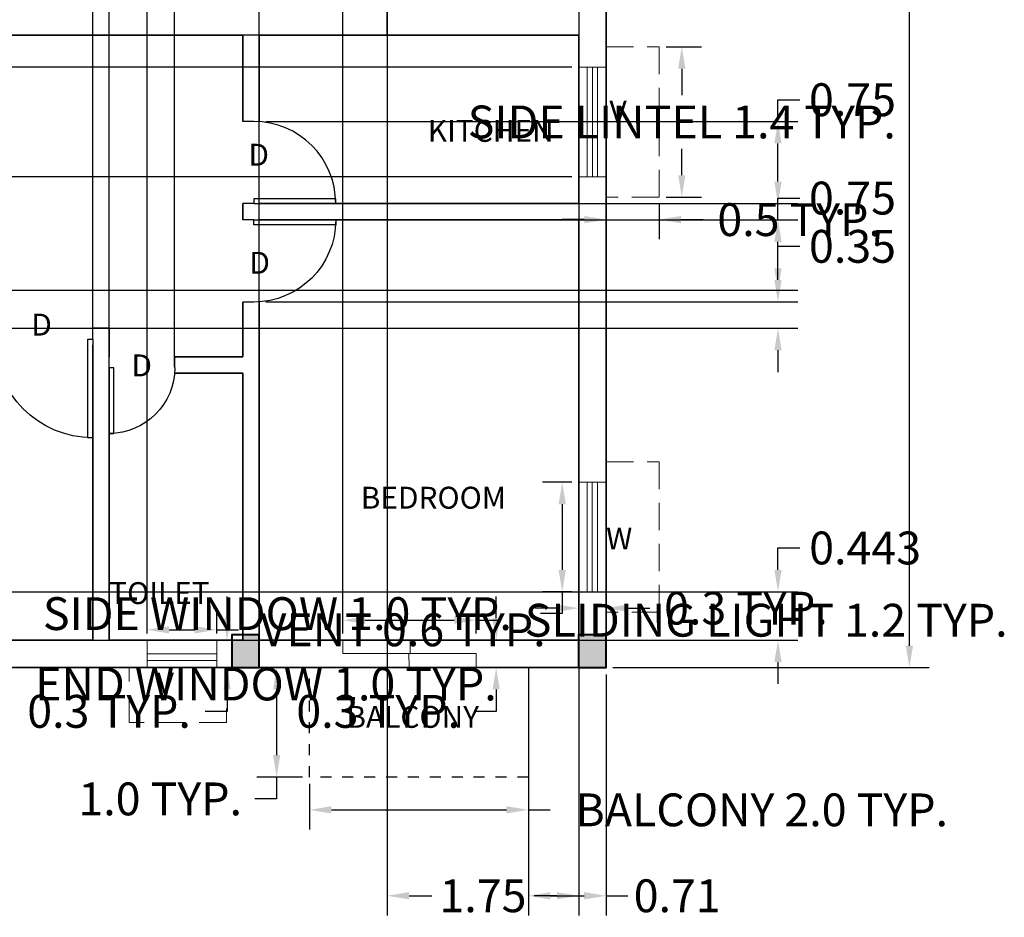
# Model space of a CAD drawing. Units: metres. Extents: x 106.5 to 121.4, y 89.1 to 111.8.
# Tile 2 of 5: x 112.4 to 121.4, y 89.1 to 97.3. Entities that reach past the tile are written whole.
import ezdxf

# ---------------------------------------------------------------- set-up
doc = ezdxf.new("R2010")
doc.units = ezdxf.units.M
doc.header["$MEASUREMENT"] = 0
doc.linetypes.add('ACAD_ISO07W100', pattern=[3, 0, -3])
doc.linetypes.add('HIDDEN', pattern=[0.375, 0.25, -0.125])
doc.layers.get('0').update_dxf_attribs({"color": 1})
for name, color, linetype, lineweight in [('A-ANNO-DIMS', 5, 'Continuous', 18), ('A-ANNO-TEXT', 4, 'Continuous', 18), ('A-AREA-IDEN', 4, 'Continuous', 18), ('A-COLS-PATT', 18, 'Continuous', 13), ('A-FLOR-BALC', 240, 'ACAD_ISO07W100', 25), ('A-WALL', 1, 'Continuous', 35), ('COLUMN', 244, 'Continuous', 40), ('DR', 2, 'Continuous', 25), ('LNTL', 240, 'HIDDEN', 18), ('VNTLTR', 8, 'Continuous', 18), ('WNDW', 3, 'Continuous', 18)]:
    doc.layers.add(name, color=color, linetype=linetype, lineweight=lineweight)
doc.styles.get("Standard").update_dxf_attribs({"font": 'arial.ttf'})
doc.dimstyles.get("Standard").update_dxf_attribs({"dimtxt": 0.3, "dimasz": 0.2, "dimexe": 0.18, "dimexo": 0.0625, "dimgap": 0.09, "dimtad": 0, "dimtih": 1, "dimtoh": 1, "dimdec": 1, "dimzin": 0, "dimdsep": 46, "dimtxsty": 'Standard', "dimcen": 0.09, "dimadec": 0, "dimazin": 0, "dimtfac": 1, "dimtdec": 1, "dimtofl": 0, "dimtmove": 0, "dimatfit": 3, "dimfxl": 1, "dimtolj": 1, "dimtzin": 0, "dimarcsym": 0})

# ---------------------------------------------------------------- blocks, each defined once
blk = doc.blocks.new('*U2')
for p, q in [((0, 0), (0, -100)), ((-900, 0), (-900, -100))]:
    blk.add_line(p, q)
blk.add_lwpolyline([(0, 0), (0, 900), (-43.75, 900), (-43.75, 0)], close=True)
blk.add_arc((0, 0), 900, 90, 180)
blk = doc.blocks.new('*U3')
for p, q in [((0, 0), (0, -100)), ((600, 0), (600, -100))]:
    blk.add_line(p, q)
blk.add_lwpolyline([(0, 0), (0, 600), (43.75, 600), (43.75, 0)], close=True)
blk.add_arc((0, 0), 600, 0, 90)
blk = doc.blocks.new('*U4')
for p, q in [((-750, 0), (-750, -100)), ((0, 0), (0, -100))]:
    blk.add_line(p, q)
blk.add_lwpolyline([(0, 0), (0, 750), (-43.75, 750), (-43.75, 0)], close=True)
blk.add_arc((0, 0), 750, 90, 180)
blk = doc.blocks.new('*D24')
at = {"layer": 'A-ANNO-DIMS', "color": 0, "lineweight": -2, "ltscale": 0.5, "transparency": 16777216}
for p, q in [((117.8454, 109.5038), (120.7343, 109.5038)), ((120.5543, 109.3038), (120.5543, 100.662)), ((120.5543, 91.5338), (120.5543, 100.1756)), ((117.8446, 91.3338), (120.7343, 91.3338))]:
    blk.add_line(p, q, dxfattribs=at)
at = {"layer": 'A-ANNO-DIMS', "color": 0, "lineweight": -3, "ltscale": 0.5, "transparency": 16777216}
for points in [[(120.521, 109.3038), (120.5876, 109.3038), (120.5543, 109.5038)], [(120.521, 91.5338), (120.5876, 91.5338), (120.5543, 91.3338)]]:
    blk.add_solid(points, dxfattribs=at)
at = {"layer": 'Defpoints', "color": 0, "lineweight": -3, "ltscale": 0.5, "transparency": 16777216}
for p in [(117.7829, 109.5038), (117.7821, 91.3338), (120.5543, 91.3338)]:
    blk.add_point(p, dxfattribs=at)
at = {"layer": 'A-ANNO-DIMS', "color": 0, "ltscale": 0.5, "transparency": 16777216, "insert": (120.5543, 100.4188), "char_height": 0.3, "attachment_point": 5}
blk.add_mtext('\\A1;18.2', dxfattribs=at)
blk = doc.blocks.new('WIN-1000-SIDE')
for p, q in [((0.0782, 0.9998), (0.0782, -0.0002)), ((0.1249, 0.9998), (0.1249, -0.0002)), ((0.1718, -0.0002), (0.1718, 0.9998))]:
    blk.add_line(p, q)
blk.add_lwpolyline([(-0.0001, 0.9998), (0.2499, 0.9998), (0.2499, -0.0002), (-0.0001, -0.0002)], close=True)
blk = doc.blocks.new('BALCONY-SLIDING-LIGHT')
for points in [[(0.6038, 0.2498), (1.217, 0.2498), (1.217, 0.1224), (0.6014, 0.1224)], [(-0.0001, -0.0002), (0.613, -0.0002), (0.613, 0.1224), (-0.0001, 0.1224)]]:
    blk.add_lwpolyline(points, close=True)
blk = doc.blocks.new('VENT-0634')
for p, q in [((-0.0005, 0.1839), (0.6339, 0.1839)), ((-0.0005, 0.1248), (0.6339, 0.1248))]:
    blk.add_line(p, q)
blk.add_lwpolyline([(-0.0005, 0.2498), (0.6339, 0.2498), (0.6339, -0.0002), (-0.0005, -0.0002)], close=True)
blk = doc.blocks.new('LINTEL-PROJ-1373')
for p, q in [((-0.0001, 1.3733), (0.4855, 1.3733)), ((0.4855, 1.3733), (0.4855, 0.0001)), ((0.4855, 0.0001), (-0.0001, 0.0001))]:
    blk.add_line(p, q)
blk = doc.blocks.new('LINTEL-PROJ-0890')
for p, q in [((0.0002, -0.0002), (0.0002, 0.5015)), ((0.0002, 0.5015), (0.8897, 0.5015)), ((0.8897, 0.5015), (0.8897, -0.0002))]:
    blk.add_line(p, q)
blk = doc.blocks.new('BALCONY-2000X1000')
at = {"ltscale": 0.02}
blk.add_lwpolyline([(-0.0001, -0.0002), (1.9999, -0.0002), (1.9999, 0.9998), (-0.0001, 0.9998)], close=True, dxfattribs=at)
blk = doc.blocks.new('COL-250X300')
at = {"ltscale": 0.5}
blk.add_lwpolyline([(-0.0001, 0.2999), (0.2499, 0.2999), (0.2499, -0.0001), (-0.0001, -0.0001)], close=True, dxfattribs=at)
blk = doc.blocks.new('*D38')
at = {"layer": 'A-ANNO-DIMS', "color": 0, "lineweight": -2, "ltscale": 0.5, "transparency": 16777216}
for p, q in [((117.4697, 93.0268), (117.2022, 93.0268)), ((117.3822, 92.8268), (117.3822, 92.2268)), ((117.4697, 92.0268), (117.2022, 92.0268)), ((117.3822, 92.0268), (117.3822, 91.8268)), ((117.3822, 91.8268), (117.1822, 91.8268))]:
    blk.add_line(p, q, dxfattribs=at)
at = {"layer": 'A-ANNO-DIMS', "color": 0, "lineweight": -3, "ltscale": 0.5, "transparency": 16777216}
for points in [[(117.3488, 92.8268), (117.4155, 92.8268), (117.3822, 93.0268)], [(117.3488, 92.2268), (117.4155, 92.2268), (117.3822, 92.0268)]]:
    blk.add_solid(points, dxfattribs=at)
at = {"layer": 'Defpoints', "color": 0, "lineweight": -3, "ltscale": 0.5, "transparency": 16777216}
for p in [(117.5322, 93.0268), (117.3822, 92.0268), (117.5322, 92.0268)]:
    blk.add_point(p, dxfattribs=at)
at = {"layer": 'A-ANNO-DIMS', "color": 0, "ltscale": 0.5, "transparency": 16777216, "insert": (114.7795, 91.8268), "char_height": 0.3, "attachment_point": 5}
blk.add_mtext('\\A1;SIDE WINDOW 1.0 TYP.', dxfattribs=at)
blk = doc.blocks.new('*D39')
at = {"layer": 'A-ANNO-DIMS', "color": 0, "lineweight": -2, "ltscale": 0.5, "transparency": 16777216}
for p, q in [((117.5322, 91.9643), (117.5322, 91.6968)), ((117.7822, 91.9643), (117.7822, 91.6968)), ((117.3322, 91.8768), (117.1322, 91.8768)), ((117.9822, 91.8768), (118.1822, 91.8768))]:
    blk.add_line(p, q, dxfattribs=at)
at = {"layer": 'A-ANNO-DIMS', "color": 0, "lineweight": -3, "ltscale": 0.5, "transparency": 16777216}
for points in [[(117.3322, 91.9101), (117.3322, 91.8434), (117.5322, 91.8768)], [(117.9822, 91.9101), (117.9822, 91.8434), (117.7822, 91.8768)]]:
    blk.add_solid(points, dxfattribs=at)
at = {"layer": 'Defpoints', "color": 0, "lineweight": -3, "ltscale": 0.5, "transparency": 16777216}
for p in [(117.5322, 92.0268), (117.7822, 92.0268), (117.7822, 91.8768)]:
    blk.add_point(p, dxfattribs=at)
at = {"layer": 'A-ANNO-DIMS', "color": 0, "ltscale": 0.5, "transparency": 16777216, "insert": (119.0605, 91.8768), "char_height": 0.3, "attachment_point": 5}
blk.add_mtext('\\A1;0.3 TYP.', dxfattribs=at)
blk = doc.blocks.new('*D40')
at = {"layer": 'A-ANNO-DIMS', "color": 0, "lineweight": -2, "ltscale": 0.5, "transparency": 16777216}
for p, q in [((111.1267, 91.2713), (111.1267, 91.0038)), ((112.1267, 91.2713), (112.1267, 91.0038)), ((111.3267, 91.1838), (111.9267, 91.1838)), ((112.1267, 91.1838), (112.3267, 91.1838))]:
    blk.add_line(p, q, dxfattribs=at)
at = {"layer": 'A-ANNO-DIMS', "color": 0, "lineweight": -3, "ltscale": 0.5, "transparency": 16777216}
for points in [[(111.3267, 91.2171), (111.3267, 91.1505), (111.1267, 91.1838)], [(111.9267, 91.2171), (111.9267, 91.1505), (112.1267, 91.1838)]]:
    blk.add_solid(points, dxfattribs=at)
at = {"layer": 'Defpoints', "color": 0, "lineweight": -3, "ltscale": 0.5, "transparency": 16777216}
for p in [(111.1267, 91.3338), (112.1267, 91.3338), (112.1267, 91.1838)]:
    blk.add_point(p, dxfattribs=at)
at = {"layer": 'A-ANNO-DIMS', "color": 0, "ltscale": 0.5, "transparency": 16777216, "insert": (114.6755, 91.1838), "char_height": 0.3, "attachment_point": 5}
blk.add_mtext('\\A1;END WINDOW 1.0 TYP.', dxfattribs=at)
blk = doc.blocks.new('*D44')
at = {"layer": 'A-ANNO-DIMS', "color": 0, "lineweight": -2, "ltscale": 0.5, "transparency": 16777216}
for p, q in [((115.3789, 91.6463), (115.3789, 91.9464)), ((116.596, 91.6463), (116.596, 91.9464)), ((115.5789, 91.7664), (116.396, 91.7664)), ((116.596, 91.7664), (116.796, 91.7664))]:
    blk.add_line(p, q, dxfattribs=at)
at = {"layer": 'A-ANNO-DIMS', "color": 0, "lineweight": -3, "ltscale": 0.5, "transparency": 16777216}
for points in [[(115.5789, 91.7997), (115.5789, 91.733), (115.3789, 91.7664)], [(116.396, 91.7997), (116.396, 91.733), (116.596, 91.7664)]]:
    blk.add_solid(points, dxfattribs=at)
at = {"layer": 'Defpoints', "color": 0, "lineweight": -3, "ltscale": 0.5, "transparency": 16777216}
for p in [(116.596, 91.7664), (115.3789, 91.5838), (116.596, 91.5838)]:
    blk.add_point(p, dxfattribs=at)
at = {"layer": 'A-ANNO-DIMS', "color": 0, "ltscale": 0.5, "transparency": 16777216, "insert": (119.2456, 91.7664), "char_height": 0.3, "attachment_point": 5}
blk.add_mtext('\\A1;SLIDING LIGHT 1.2 TYP.', dxfattribs=at)
blk = doc.blocks.new('*D45')
at = {"layer": 'A-ANNO-DIMS', "color": 0, "lineweight": -2, "ltscale": 0.5, "transparency": 16777216}
for p, q in [((116.7785, 91.7838), (116.7785, 91.9838)), ((116.6585, 91.5838), (116.9585, 91.5838)), ((116.6585, 91.3338), (116.9585, 91.3338)), ((116.7785, 91.1338), (116.7785, 90.9338)), ((116.7785, 90.9338), (116.5785, 90.9338))]:
    blk.add_line(p, q, dxfattribs=at)
at = {"layer": 'A-ANNO-DIMS', "color": 0, "lineweight": -3, "ltscale": 0.5, "transparency": 16777216}
for points in [[(116.7452, 91.7838), (116.8119, 91.7838), (116.7785, 91.5838)], [(116.7452, 91.1338), (116.8119, 91.1338), (116.7785, 91.3338)]]:
    blk.add_solid(points, dxfattribs=at)
at = {"layer": 'Defpoints', "color": 0, "lineweight": -3, "ltscale": 0.5, "transparency": 16777216}
for p in [(116.596, 91.5838), (116.596, 91.3338), (116.7785, 91.3338)]:
    blk.add_point(p, dxfattribs=at)
at = {"layer": 'A-ANNO-DIMS', "color": 0, "ltscale": 0.5, "transparency": 16777216, "insert": (115.7002, 90.9338), "char_height": 0.3, "attachment_point": 5}
blk.add_mtext('\\A1;0.3 TYP.', dxfattribs=at)
blk = doc.blocks.new('*D46')
at = {"layer": 'A-ANNO-DIMS', "color": 0, "lineweight": -2, "ltscale": 0.5, "transparency": 16777216}
for p, q in [((113.5905, 91.6463), (113.5905, 91.859)), ((114.2249, 91.6463), (114.2249, 91.859)), ((113.7905, 91.679), (114.0249, 91.679)), ((114.2249, 91.679), (114.4249, 91.679))]:
    blk.add_line(p, q, dxfattribs=at)
at = {"layer": 'A-ANNO-DIMS', "color": 0, "lineweight": -3, "ltscale": 0.5, "transparency": 16777216}
for points in [[(113.7905, 91.7123), (113.7905, 91.6456), (113.5905, 91.679)], [(114.0249, 91.7123), (114.0249, 91.6456), (114.2249, 91.679)]]:
    blk.add_solid(points, dxfattribs=at)
at = {"layer": 'Defpoints', "color": 0, "lineweight": -3, "ltscale": 0.5, "transparency": 16777216}
for p in [(114.2249, 91.679), (113.5905, 91.5838), (114.2249, 91.5838)]:
    blk.add_point(p, dxfattribs=at)
at = {"layer": 'A-ANNO-DIMS', "color": 0, "ltscale": 0.5, "transparency": 16777216, "insert": (115.9281, 91.679), "char_height": 0.3, "attachment_point": 5}
blk.add_mtext('\\A1;VENT 0.6 TYP.', dxfattribs=at)
blk = doc.blocks.new('*D47')
at = {"layer": 'A-ANNO-DIMS', "color": 0, "lineweight": -2, "ltscale": 0.5, "transparency": 16777216}
for p, q in [((114.32, 91.7838), (114.32, 91.9838)), ((114.2874, 91.5838), (114.5, 91.5838)), ((114.2874, 91.3338), (114.5, 91.3338)), ((114.32, 91.1338), (114.32, 90.9338)), ((114.32, 90.9338), (114.12, 90.9338))]:
    blk.add_line(p, q, dxfattribs=at)
at = {"layer": 'A-ANNO-DIMS', "color": 0, "lineweight": -3, "ltscale": 0.5, "transparency": 16777216}
for points in [[(114.2867, 91.7838), (114.3534, 91.7838), (114.32, 91.5838)], [(114.2867, 91.1338), (114.3534, 91.1338), (114.32, 91.3338)]]:
    blk.add_solid(points, dxfattribs=at)
at = {"layer": 'Defpoints', "color": 0, "lineweight": -3, "ltscale": 0.5, "transparency": 16777216}
for p in [(114.2249, 91.5838), (114.2249, 91.3338), (114.32, 91.3338)]:
    blk.add_point(p, dxfattribs=at)
at = {"layer": 'A-ANNO-DIMS', "color": 0, "ltscale": 0.5, "transparency": 16777216, "insert": (113.2417, 90.9338), "char_height": 0.3, "attachment_point": 5}
blk.add_mtext('\\A1;0.3 TYP.', dxfattribs=at)
blk = doc.blocks.new('*D50')
at = {"layer": 'A-ANNO-DIMS', "color": 0, "lineweight": -2, "ltscale": 0.5, "transparency": 16777216}
for p, q in [((118.331, 97.0058), (118.6544, 97.0058)), ((118.4744, 96.8058), (118.4744, 96.5644)), ((118.4744, 95.8327), (118.4744, 96.0742)), ((118.331, 95.6327), (118.6544, 95.6327))]:
    blk.add_line(p, q, dxfattribs=at)
at = {"layer": 'A-ANNO-DIMS', "color": 0, "lineweight": -3, "ltscale": 0.5, "transparency": 16777216}
for points in [[(118.4411, 96.8058), (118.5078, 96.8058), (118.4744, 97.0058)], [(118.4411, 95.8327), (118.5078, 95.8327), (118.4744, 95.6327)]]:
    blk.add_solid(points, dxfattribs=at)
at = {"layer": 'Defpoints', "color": 0, "lineweight": -3, "ltscale": 0.5, "transparency": 16777216}
for p in [(118.2685, 97.0058), (118.4744, 97.0058), (118.2685, 95.6327)]:
    blk.add_point(p, dxfattribs=at)
at = {"layer": 'A-ANNO-DIMS', "color": 0, "ltscale": 0.5, "transparency": 16777216, "insert": (118.4744, 96.3193), "char_height": 0.3, "attachment_point": 5}
blk.add_mtext('\\A1;SIDE LINTEL 1.4 TYP.', dxfattribs=at)
blk = doc.blocks.new('*D51')
at = {"layer": 'A-ANNO-DIMS', "color": 0, "lineweight": -2, "ltscale": 0.5, "transparency": 16777216}
for p, q in [((117.7829, 95.5702), (117.7829, 95.2468)), ((118.2685, 95.5702), (118.2685, 95.2468)), ((117.5829, 95.4268), (117.3829, 95.4268)), ((118.4685, 95.4268), (118.6685, 95.4268))]:
    blk.add_line(p, q, dxfattribs=at)
at = {"layer": 'A-ANNO-DIMS', "color": 0, "lineweight": -3, "ltscale": 0.5, "transparency": 16777216}
for points in [[(117.5829, 95.4601), (117.5829, 95.3934), (117.7829, 95.4268)], [(118.4685, 95.4601), (118.4685, 95.3934), (118.2685, 95.4268)]]:
    blk.add_solid(points, dxfattribs=at)
at = {"layer": 'Defpoints', "color": 0, "lineweight": -3, "ltscale": 0.5, "transparency": 16777216}
for p in [(117.7829, 95.6327), (118.2685, 95.6327), (118.2685, 95.4268)]:
    blk.add_point(p, dxfattribs=at)
at = {"layer": 'A-ANNO-DIMS', "color": 0, "ltscale": 0.5, "transparency": 16777216, "insert": (119.5468, 95.4268), "char_height": 0.3, "attachment_point": 5}
blk.add_mtext('\\A1;0.5 TYP.', dxfattribs=at)
blk = doc.blocks.new('*D56')
at = {"layer": 'A-ANNO-DIMS', "color": 0, "lineweight": -2, "ltscale": 0.5, "transparency": 16777216}
for p, q in [((115.0729, 90.2713), (115.0729, 89.8538)), ((117.0729, 90.2713), (117.0729, 89.8538)), ((115.2729, 90.0338), (116.8729, 90.0338)), ((117.0729, 90.0338), (117.2729, 90.0338))]:
    blk.add_line(p, q, dxfattribs=at)
at = {"layer": 'A-ANNO-DIMS', "color": 0, "lineweight": -3, "ltscale": 0.5, "transparency": 16777216}
for points in [[(115.2729, 90.0671), (115.2729, 90.0005), (115.0729, 90.0338)], [(116.8729, 90.0671), (116.8729, 90.0005), (117.0729, 90.0338)]]:
    blk.add_solid(points, dxfattribs=at)
at = {"layer": 'Defpoints', "color": 0, "lineweight": -3, "ltscale": 0.5, "transparency": 16777216}
for p in [(115.0729, 90.3338), (117.0729, 90.3338), (117.0729, 90.0338)]:
    blk.add_point(p, dxfattribs=at)
at = {"layer": 'A-ANNO-DIMS', "color": 0, "ltscale": 0.5, "transparency": 16777216, "insert": (119.2044, 90.0338), "char_height": 0.3, "attachment_point": 5}
blk.add_mtext('\\A1;BALCONY 2.0 TYP.', dxfattribs=at)
blk = doc.blocks.new('*D57')
at = {"layer": 'A-ANNO-DIMS', "color": 0, "lineweight": -2, "ltscale": 0.5, "transparency": 16777216}
for p, q in [((115.0104, 91.3338), (114.5929, 91.3338)), ((114.7729, 91.1338), (114.7729, 90.5338)), ((115.0104, 90.3338), (114.5929, 90.3338)), ((114.7729, 90.3338), (114.7729, 90.1338)), ((114.7729, 90.1338), (114.5729, 90.1338))]:
    blk.add_line(p, q, dxfattribs=at)
at = {"layer": 'A-ANNO-DIMS', "color": 0, "lineweight": -3, "ltscale": 0.5, "transparency": 16777216}
for points in [[(114.7396, 91.1338), (114.8063, 91.1338), (114.7729, 91.3338)], [(114.7396, 90.5338), (114.8063, 90.5338), (114.7729, 90.3338)]]:
    blk.add_solid(points, dxfattribs=at)
at = {"layer": 'Defpoints', "color": 0, "lineweight": -3, "ltscale": 0.5, "transparency": 16777216}
for p in [(115.0729, 91.3338), (114.7729, 90.3338), (115.0729, 90.3338)]:
    blk.add_point(p, dxfattribs=at)
at = {"layer": 'A-ANNO-DIMS', "color": 0, "ltscale": 0.5, "transparency": 16777216, "insert": (113.7087, 90.1338), "char_height": 0.3, "attachment_point": 5}
blk.add_mtext('\\A1;1.0 TYP.', dxfattribs=at)
blk = doc.blocks.new('*D59')
at = {"layer": 'A-ANNO-DIMS', "color": 0, "lineweight": -2, "ltscale": 0.5, "transparency": 16777216}
for p, q in [((112.1943, 94.3463), (112.1943, 111.7688)), ((113.0929, 94.3463), (113.0929, 111.7688)), ((112.3943, 111.5888), (112.8929, 111.5888)), ((113.0929, 111.5888), (113.2929, 111.5888))]:
    blk.add_line(p, q, dxfattribs=at)
at = {"layer": 'A-ANNO-DIMS', "color": 0, "lineweight": -3, "ltscale": 0.5, "transparency": 16777216}
for points in [[(112.3943, 111.6221), (112.3943, 111.5555), (112.1943, 111.5888)], [(112.8929, 111.6221), (112.8929, 111.5555), (113.0929, 111.5888)]]:
    blk.add_solid(points, dxfattribs=at)
at = {"layer": 'Defpoints', "color": 0, "lineweight": -3, "ltscale": 0.5, "transparency": 16777216}
for p in [(113.0929, 111.5888), (112.1943, 94.2838), (113.0929, 94.2838)]:
    blk.add_point(p, dxfattribs=at)
at = {"layer": 'A-ANNO-DIMS', "color": 0, "ltscale": 0.5, "transparency": 16777216, "insert": (113.772, 111.5888), "char_height": 0.3, "attachment_point": 5}
blk.add_mtext('\\A1;0.90', dxfattribs=at)
blk = doc.blocks.new('*D60')
at = {"layer": 'A-ANNO-DIMS', "color": 0, "lineweight": -2, "ltscale": 0.5, "transparency": 16777216}
for p, q in [((113.2429, 94.0863), (113.2429, 111.7688)), ((113.8408, 94.0863), (113.8408, 111.7688)), ((113.4429, 111.5888), (113.6408, 111.5888)), ((113.8408, 111.5888), (114.0408, 111.5888))]:
    blk.add_line(p, q, dxfattribs=at)
at = {"layer": 'A-ANNO-DIMS', "color": 0, "lineweight": -3, "ltscale": 0.5, "transparency": 16777216}
for points in [[(113.4429, 111.6221), (113.4429, 111.5555), (113.2429, 111.5888)], [(113.6408, 111.6221), (113.6408, 111.5555), (113.8408, 111.5888)]]:
    blk.add_solid(points, dxfattribs=at)
at = {"layer": 'Defpoints', "color": 0, "lineweight": -3, "ltscale": 0.5, "transparency": 16777216}
for p in [(113.8408, 111.5888), (113.2429, 94.0238), (113.8408, 94.0238)]:
    blk.add_point(p, dxfattribs=at)
at = {"layer": 'A-ANNO-DIMS', "color": 0, "ltscale": 0.5, "transparency": 16777216, "insert": (114.6373, 111.5888), "char_height": 0.3, "attachment_point": 5}
blk.add_mtext('\\A1;0.598', dxfattribs=at)
blk = doc.blocks.new('*D61')
at = {"layer": 'A-ANNO-DIMS', "color": 0, "lineweight": -2, "ltscale": 0.5, "transparency": 16777216}
for p, q in [((119.3535, 95.4238), (119.3535, 95.6238)), ((119.3535, 95.6238), (119.5535, 95.6238)), ((114.6754, 95.4238), (119.5335, 95.4238)), ((119.3535, 94.8755), (119.3535, 95.2238)), ((114.6754, 94.6755), (119.5335, 94.6755))]:
    blk.add_line(p, q, dxfattribs=at)
at = {"layer": 'A-ANNO-DIMS', "color": 0, "lineweight": -3, "ltscale": 0.5, "transparency": 16777216}
for points in [[(119.3201, 95.2238), (119.3868, 95.2238), (119.3535, 95.4238)], [(119.3201, 94.8755), (119.3868, 94.8755), (119.3535, 94.6755)]]:
    blk.add_solid(points, dxfattribs=at)
at = {"layer": 'Defpoints', "color": 0, "lineweight": -3, "ltscale": 0.5, "transparency": 16777216}
for p in [(114.6129, 95.4238), (119.3535, 95.4238), (114.6129, 94.6755)]:
    blk.add_point(p, dxfattribs=at)
at = {"layer": 'A-ANNO-DIMS', "color": 0, "ltscale": 0.5, "transparency": 16777216, "insert": (120.0342, 95.6238), "char_height": 0.3, "attachment_point": 5}
blk.add_mtext('\\A1;0.75', dxfattribs=at)
blk = doc.blocks.new('*D62')
at = {"layer": 'A-ANNO-DIMS', "color": 0, "lineweight": -2, "ltscale": 0.5, "transparency": 16777216}
for p, q in [((119.3535, 96.3225), (119.3535, 96.5225)), ((119.3535, 96.5225), (119.5535, 96.5225)), ((114.6754, 96.3225), (119.5335, 96.3225)), ((119.3535, 95.7738), (119.3535, 96.1225)), ((114.6754, 95.5738), (119.5335, 95.5738))]:
    blk.add_line(p, q, dxfattribs=at)
at = {"layer": 'A-ANNO-DIMS', "color": 0, "lineweight": -3, "ltscale": 0.5, "transparency": 16777216}
for points in [[(119.3201, 96.1225), (119.3868, 96.1225), (119.3535, 96.3225)], [(119.3201, 95.7738), (119.3868, 95.7738), (119.3535, 95.5738)]]:
    blk.add_solid(points, dxfattribs=at)
at = {"layer": 'Defpoints', "color": 0, "lineweight": -3, "ltscale": 0.5, "transparency": 16777216}
for p in [(114.6129, 96.3225), (119.3535, 96.3225), (114.6129, 95.5738)]:
    blk.add_point(p, dxfattribs=at)
at = {"layer": 'A-ANNO-DIMS', "color": 0, "ltscale": 0.5, "transparency": 16777216, "insert": (120.0342, 96.5225), "char_height": 0.3, "attachment_point": 5}
blk.add_mtext('\\A1;0.75', dxfattribs=at)
blk = doc.blocks.new('*D64')
at = {"layer": 'A-ANNO-DIMS', "color": 0, "lineweight": -2, "ltscale": 0.5, "transparency": 16777216}
for p, q in [((113.2429, 91.6463), (113.2429, 111.7688)), ((113.5905, 91.6463), (113.5905, 111.7688)), ((113.0429, 111.5888), (112.8429, 111.5888)), ((113.7905, 111.5888), (113.9905, 111.5888))]:
    blk.add_line(p, q, dxfattribs=at)
at = {"layer": 'A-ANNO-DIMS', "color": 0, "lineweight": -3, "ltscale": 0.5, "transparency": 16777216}
for points in [[(113.0429, 111.6221), (113.0429, 111.5555), (113.2429, 111.5888)], [(113.7905, 111.6221), (113.7905, 111.5555), (113.5905, 111.5888)]]:
    blk.add_solid(points, dxfattribs=at)
at = {"layer": 'Defpoints', "color": 0, "lineweight": -3, "ltscale": 0.5, "transparency": 16777216}
for p in [(113.5905, 111.5888), (113.2429, 91.5838), (113.5905, 91.5838)]:
    blk.add_point(p, dxfattribs=at)
at = {"layer": 'A-ANNO-DIMS', "color": 0, "ltscale": 0.5, "transparency": 16777216, "insert": (114.4713, 111.5888), "char_height": 0.3, "attachment_point": 5}
blk.add_mtext('\\A1;0.35', dxfattribs=at)
blk = doc.blocks.new('*D65')
at = {"layer": 'A-ANNO-DIMS', "color": 0, "lineweight": -2, "ltscale": 0.5, "transparency": 16777216}
for p, q in [((114.6129, 91.6463), (114.6129, 111.7688)), ((115.3789, 91.6463), (115.3789, 111.7688)), ((114.8129, 111.5888), (115.1789, 111.5888)), ((115.3789, 111.5888), (115.5789, 111.5888))]:
    blk.add_line(p, q, dxfattribs=at)
at = {"layer": 'A-ANNO-DIMS', "color": 0, "lineweight": -3, "ltscale": 0.5, "transparency": 16777216}
for points in [[(114.8129, 111.6221), (114.8129, 111.5555), (114.6129, 111.5888)], [(115.1789, 111.6221), (115.1789, 111.5555), (115.3789, 111.5888)]]:
    blk.add_solid(points, dxfattribs=at)
at = {"layer": 'Defpoints', "color": 0, "lineweight": -3, "ltscale": 0.5, "transparency": 16777216}
for p in [(115.3789, 111.5888), (114.6129, 91.5838), (115.3789, 91.5838)]:
    blk.add_point(p, dxfattribs=at)
at = {"layer": 'A-ANNO-DIMS', "color": 0, "ltscale": 0.5, "transparency": 16777216, "insert": (116.1749, 111.5888), "char_height": 0.3, "attachment_point": 5}
blk.add_mtext('\\A1;0.766', dxfattribs=at)
blk = doc.blocks.new('*D66')
at = {"layer": 'A-ANNO-DIMS', "color": 0, "lineweight": -2, "ltscale": 0.5, "transparency": 16777216}
for p, q in [((117.0729, 91.2713), (117.0729, 89.0688)), ((117.7821, 91.2713), (117.7821, 89.0688)), ((117.2729, 89.2488), (117.5821, 89.2488)), ((117.7821, 89.2488), (117.9821, 89.2488))]:
    blk.add_line(p, q, dxfattribs=at)
at = {"layer": 'A-ANNO-DIMS', "color": 0, "lineweight": -3, "ltscale": 0.5, "transparency": 16777216}
for points in [[(117.2729, 89.2821), (117.2729, 89.2155), (117.0729, 89.2488)], [(117.5821, 89.2821), (117.5821, 89.2155), (117.7821, 89.2488)]]:
    blk.add_solid(points, dxfattribs=at)
at = {"layer": 'Defpoints', "color": 0, "lineweight": -3, "ltscale": 0.5, "transparency": 16777216}
for p in [(117.0729, 91.3338), (117.7821, 91.3338), (117.7821, 89.2488)]:
    blk.add_point(p, dxfattribs=at)
at = {"layer": 'A-ANNO-DIMS', "color": 0, "ltscale": 0.5, "transparency": 16777216, "insert": (118.4328, 89.2488), "char_height": 0.3, "attachment_point": 5}
blk.add_mtext('\\A1;0.71', dxfattribs=at)
blk = doc.blocks.new('*D67')
at = {"layer": 'A-ANNO-DIMS', "color": 0, "lineweight": -2, "ltscale": 0.5, "transparency": 16777216}
for p, q in [((119.3535, 92.2268), (119.3535, 92.4268)), ((119.3535, 92.4268), (119.5535, 92.4268)), ((110.5154, 92.0268), (119.5335, 92.0268)), ((110.5154, 91.5838), (119.5335, 91.5838)), ((119.3535, 91.3838), (119.3535, 91.1838))]:
    blk.add_line(p, q, dxfattribs=at)
at = {"layer": 'A-ANNO-DIMS', "color": 0, "lineweight": -3, "ltscale": 0.5, "transparency": 16777216}
for points in [[(119.3201, 92.2268), (119.3868, 92.2268), (119.3535, 92.0268)], [(119.3201, 91.3838), (119.3868, 91.3838), (119.3535, 91.5838)]]:
    blk.add_solid(points, dxfattribs=at)
at = {"layer": 'Defpoints', "color": 0, "lineweight": -3, "ltscale": 0.5, "transparency": 16777216}
for p in [(110.4529, 92.0268), (119.3535, 92.0268), (110.4529, 91.5838)]:
    blk.add_point(p, dxfattribs=at)
at = {"layer": 'A-ANNO-DIMS', "color": 0, "ltscale": 0.5, "transparency": 16777216, "insert": (120.1496, 92.4268), "char_height": 0.3, "attachment_point": 5}
blk.add_mtext('\\A1;0.443', dxfattribs=at)
blk = doc.blocks.new('*D68')
at = {"layer": 'A-ANNO-DIMS', "color": 0, "lineweight": -2, "ltscale": 0.5, "transparency": 16777216}
for p, q in [((119.3535, 94.9829), (119.3535, 95.1829)), ((119.3535, 95.1829), (119.5535, 95.1829)), ((110.5154, 94.7829), (119.5335, 94.7829)), ((110.5154, 94.4338), (119.5335, 94.4338)), ((119.3535, 94.2338), (119.3535, 94.0338))]:
    blk.add_line(p, q, dxfattribs=at)
at = {"layer": 'A-ANNO-DIMS', "color": 0, "lineweight": -3, "ltscale": 0.5, "transparency": 16777216}
for points in [[(119.3201, 94.9829), (119.3868, 94.9829), (119.3535, 94.7829)], [(119.3201, 94.2338), (119.3868, 94.2338), (119.3535, 94.4338)]]:
    blk.add_solid(points, dxfattribs=at)
at = {"layer": 'Defpoints', "color": 0, "lineweight": -3, "ltscale": 0.5, "transparency": 16777216}
for p in [(110.4529, 94.7829), (119.3535, 94.7829), (110.4529, 94.4338)]:
    blk.add_point(p, dxfattribs=at)
at = {"layer": 'A-ANNO-DIMS', "color": 0, "ltscale": 0.5, "transparency": 16777216, "insert": (120.0342, 95.1829), "char_height": 0.3, "attachment_point": 5}
blk.add_mtext('\\A1;0.35', dxfattribs=at)
blk = doc.blocks.new('*D69')
at = {"layer": 'A-ANNO-DIMS', "color": 0, "lineweight": -2, "ltscale": 0.5, "transparency": 16777216}
for p, q in [((108.4073, 97.3137), (108.4073, 97.5137)), ((108.4073, 97.5137), (108.6073, 97.5137)), ((117.4704, 97.1137), (108.2273, 97.1137)), ((117.4697, 96.8192), (108.2273, 96.8192)), ((108.4073, 96.6192), (108.4073, 96.4192))]:
    blk.add_line(p, q, dxfattribs=at)
at = {"layer": 'A-ANNO-DIMS', "color": 0, "lineweight": -3, "ltscale": 0.5, "transparency": 16777216}
for points in [[(108.3739, 97.3137), (108.4406, 97.3137), (108.4073, 97.1137)], [(108.3739, 96.6192), (108.4406, 96.6192), (108.4073, 96.8192)]]:
    blk.add_solid(points, dxfattribs=at)
at = {"layer": 'Defpoints', "color": 0, "lineweight": -3, "ltscale": 0.5, "transparency": 16777216}
for p in [(108.4073, 97.1137), (117.5329, 97.1137), (117.5322, 96.8192)]:
    blk.add_point(p, dxfattribs=at)
at = {"layer": 'A-ANNO-DIMS', "color": 0, "ltscale": 0.5, "transparency": 16777216, "insert": (109.0872, 97.5137), "char_height": 0.3, "attachment_point": 5}
blk.add_mtext('\\A1;0.29', dxfattribs=at)
blk = doc.blocks.new('*D70')
at = {"layer": 'A-ANNO-DIMS', "color": 0, "lineweight": -2, "ltscale": 0.5, "transparency": 16777216}
for p, q in [((108.4073, 96.8192), (108.4073, 97.0191)), ((108.4073, 97.0191), (108.6073, 97.0191)), ((117.4697, 96.8192), (108.2273, 96.8192)), ((108.4073, 96.0192), (108.4073, 96.6192)), ((117.4697, 95.8192), (108.2273, 95.8192))]:
    blk.add_line(p, q, dxfattribs=at)
at = {"layer": 'A-ANNO-DIMS', "color": 0, "lineweight": -3, "ltscale": 0.5, "transparency": 16777216}
for points in [[(108.3739, 96.6192), (108.4406, 96.6192), (108.4073, 96.8192)], [(108.3739, 96.0192), (108.4406, 96.0192), (108.4073, 95.8192)]]:
    blk.add_solid(points, dxfattribs=at)
at = {"layer": 'Defpoints', "color": 0, "lineweight": -3, "ltscale": 0.5, "transparency": 16777216}
for p in [(108.4073, 96.8192), (117.5322, 96.8192), (117.5322, 95.8192)]:
    blk.add_point(p, dxfattribs=at)
at = {"layer": 'A-ANNO-DIMS', "color": 0, "ltscale": 0.5, "transparency": 16777216, "insert": (108.9557, 97.0191), "char_height": 0.3, "attachment_point": 5}
blk.add_mtext('\\A1;1.0', dxfattribs=at)
blk = doc.blocks.new('*D74')
at = {"layer": 'A-ANNO-DIMS', "color": 0, "lineweight": -2, "ltscale": 0.5, "transparency": 16777216}
for p, q in [((115.7829, 98.6813), (115.7829, 89.0688)), ((117.5329, 98.6813), (117.5329, 89.0688)), ((115.9829, 89.2488), (116.1913, 89.2488)), ((117.3329, 89.2488), (117.1246, 89.2488))]:
    blk.add_line(p, q, dxfattribs=at)
at = {"layer": 'A-ANNO-DIMS', "color": 0, "lineweight": -3, "ltscale": 0.5, "transparency": 16777216}
for points in [[(115.9829, 89.2821), (115.9829, 89.2155), (115.7829, 89.2488)], [(117.3329, 89.2821), (117.3329, 89.2155), (117.5329, 89.2488)]]:
    blk.add_solid(points, dxfattribs=at)
at = {"layer": 'Defpoints', "color": 0, "lineweight": -3, "ltscale": 0.5, "transparency": 16777216}
for p in [(115.7829, 98.7438), (117.5329, 98.7438), (117.5329, 89.2488)]:
    blk.add_point(p, dxfattribs=at)
at = {"layer": 'A-ANNO-DIMS', "color": 0, "ltscale": 0.5, "transparency": 16777216, "insert": (116.6579, 89.2488), "char_height": 0.3, "attachment_point": 5}
blk.add_mtext('\\A1;1.75', dxfattribs=at)

msp = doc.modelspace()

# ---------------------------------------------------------------- hatches: boundary and pattern name
at = {"layer": 'A-COLS-PATT', "ltscale": 0.5}
h = msp.add_hatch(color=256, dxfattribs=at)
h.dxf.hatch_style = 1
h.paths.add_polyline_path([(110.4529, 103.8929), (110.2029, 103.8929), (110.2029, 103.5938), (110.4529, 103.5938)])
h.paths.add_polyline_path([(114.4629, 103.8938), (114.3632, 103.8938), (114.3632, 103.7438), (114.4629, 103.7438)])
h.paths.add_polyline_path([(114.6129, 103.8938), (114.4629, 103.8938), (114.4629, 103.7438), (114.6129, 103.7438)])
h.paths.add_polyline_path([(114.6132, 103.7438), (114.4629, 103.7438), (114.3632, 103.7438), (114.3632, 103.5938), (114.6132, 103.5938)])
h.paths.add_polyline_path([(117.7829, 103.8996), (117.5329, 103.8996), (117.5329, 103.5996), (117.7829, 103.5996)])
h.paths.add_polyline_path([(117.7829, 98.888), (117.5329, 98.888), (117.5329, 98.588), (117.7829, 98.588)])
h.paths.add_polyline_path([(110.4529, 98.8938), (110.2029, 98.8938), (110.2029, 98.5947), (110.4529, 98.5947)])
h.paths.add_polyline_path([(114.6132, 98.8938), (114.3132, 98.8938), (114.3132, 98.7438), (114.4632, 98.7438), (114.6132, 98.7438)])
h.paths.add_polyline_path([(110.4529, 91.6338), (110.2029, 91.6338), (110.2029, 91.3338), (110.4529, 91.3338)])
h.paths.add_polyline_path([(114.6132, 91.5838), (114.6129, 91.5838), (114.6129, 91.6338), (114.4629, 91.6338), (114.4629, 91.5838), (114.3632, 91.5838), (114.3632, 91.3338), (114.6132, 91.3338)])
h.paths.add_polyline_path([(117.7821, 91.6338), (117.5329, 91.6338), (117.5329, 91.5838), (117.5321, 91.3338), (117.7821, 91.3338)])
h = msp.add_hatch(dxfattribs=at)
h.set_pattern_fill('CORK', color=256, scale=10)
h.set_pattern_definition([(0, (0, 0), (0, 1.25), []), (135, (0.625, -0.625), (-2.5, -2.5), [1.76777, -1.76777]), (135, (0.9375, -0.625), (-2.5, -2.5), [1.76777, -1.76777]), (135, (1.25, -0.625), (-2.5, -2.5), [1.76777, -1.76777])])
h.paths.add_polyline_path([(110.2029, 93.2238), (110.2029, 93.5238), (110.4529, 93.5238), (110.4529, 93.2238)])
h.paths.add_polyline_path([(114.6132, 93.2238), (114.3632, 93.2238), (114.3632, 93.4738), (114.4629, 93.4738), (114.4629, 93.5238), (114.6129, 93.5238), (114.6129, 93.4738)])
h.paths.add_polyline_path([(117.5321, 93.4738), (117.5329, 93.4738), (117.5329, 93.5238), (117.7821, 93.5238), (117.7821, 93.2238), (117.5321, 93.2238)])

# ---------------------------------------------------------------- linework, layer by layer
at = {"layer": 'A-WALL'}
for p, q in [((117.7829, 101.9438), (117.7829, 91.3338)), ((115.7829, 98.8938), (115.7829, 97.1137)), ((114.4629, 97.1137), (111.4529, 97.1137)), ((114.4629, 96.3242), (114.4629, 97.1137)), ((114.6129, 96.3225), (114.6129, 97.1137)), ((117.5329, 97.1137), (114.6129, 97.1137)), ((117.5329, 97.1137), (117.5329, 95.5738)), ((114.4629, 95.4238), (114.4629, 95.5742)), ((114.6129, 95.5738), (114.6129, 95.5742)), ((117.5329, 95.5738), (114.6129, 95.5738)), ((117.5329, 95.4238), (114.6129, 95.4238)), ((117.5329, 95.4238), (117.5329, 91.5838)), ((114.4629, 94.1738), (114.4629, 94.6738)), ((114.6129, 91.5838), (114.6129, 94.6755)), ((113.2429, 94.1738), (113.2429, 94.4338)), ((113.0929, 91.5838), (113.0929, 94.2838)), ((114.4629, 94.1738), (113.8429, 94.1738)), ((113.2429, 91.5838), (113.2429, 94.0238)), ((114.4629, 94.0238), (113.8408, 94.0238)), ((114.4629, 91.5838), (114.4629, 94.0238)), ((117.5322, 92.7838), (117.5329, 92.7838)), ((117.5322, 92.5338), (117.5329, 92.5338)), ((117.7822, 92.5338), (117.7829, 92.5338)), ((113.0929, 91.5838), (110.4529, 91.5838)), ((114.4629, 91.5838), (113.2429, 91.5838)), ((117.5329, 91.5838), (114.6129, 91.5838)), ((117.7829, 91.3338), (110.2029, 91.3338))]:
    msp.add_line(p, q, dxfattribs=at)
at = {"layer": 'A-WALL', "ltscale": 0.5}
msp.add_line((113.0929, 94.4338), (113.2429, 94.4338), dxfattribs=at)
msp.add_line((113.0929, 94.4338), (113.2429, 94.4338), dxfattribs=at)
at = {"layer": 'COLUMN', "ltscale": 0.5}
msp.add_lwpolyline([(117.5321, 91.3338), (117.7821, 91.3338), (117.7821, 91.6338), (117.5321, 91.6338)], close=True, dxfattribs=at)
at = {"layer": 'VNTLTR'}
for p, q in [((117.6105, 95.8191), (117.6105, 96.8191)), ((117.6572, 95.8191), (117.6572, 96.8191)), ((117.704, 96.8191), (117.704, 95.8191))]:
    msp.add_line(p, q, dxfattribs=at)
msp.add_lwpolyline([(117.5322, 95.8191), (117.7822, 95.8191), (117.7822, 96.8191), (117.5322, 96.8191)], close=True, dxfattribs=at)

# ---------------------------------------------------------------- block references
at = {"layer": 'A-FLOR-BALC', "extrusion": (0, 0, -1), "zscale": -1, "rotation": 180}
msp.add_blockref('BALCONY-2000X1000', (-115.073, 91.3336), dxfattribs=at)
at = {"layer": 'COLUMN', "extrusion": (0, 0, -1), "zscale": -1, "rotation": 180}
msp.add_blockref('COL-250X300', (-114.3633, 91.6337), dxfattribs=at)
at = {"layer": 'DR', "yscale": 0.001, "zscale": 0.001}
for name, p, xscale, rotation in [('*U4', (114.5629, 95.5742), 0.001, 270.0000000000015), ('*U4', (114.5629, 95.4238), -0.001, 270.0000000000015), ('*U2', (113.0929, 94.3338), -0.001, 180), ('*U3', (113.2429, 94.0738), -0.001, 180)]:
    msp.add_blockref(name, p, dxfattribs=dict(at, xscale=xscale, rotation=rotation))
at = {"layer": 'LNTL'}
for p in [(117.783, 95.6326), (117.783, 91.8402)]:
    msp.add_blockref('LINTEL-PROJ-1373', p, dxfattribs=at)
at = {"layer": 'LNTL', "rotation": 180}
msp.add_blockref('LINTEL-PROJ-0890', (114.3139, 91.3336), dxfattribs=at)
at = {"layer": 'VNTLTR', "extrusion": (0, 0, -1), "zscale": -1, "rotation": 180}
msp.add_blockref('VENT-0634', (-113.591, 91.5836), dxfattribs=at)
at = {"layer": 'WNDW', "extrusion": (0, 0, -1), "zscale": -1, "rotation": 180}
for name, p in [('WIN-1000-SIDE', (-117.5322, 93.0266)), ('BALCONY-SLIDING-LIGHT', (-115.379, 91.5836))]:
    msp.add_blockref(name, p, dxfattribs=at)

# ---------------------------------------------------------------- texts
at = {"layer": 'A-ANNO-TEXT', "ltscale": 0.5, "char_height": 0.2}
for s, width, insert, attachment_point in [('V', 0.327871, (117.8138, 96.3124), 7), ('D', 0.320447, (114.515, 96.1195), 1), ('D', 0.320447, (114.5238, 95.1325), 1), ('D', 0.320447, (112.5312, 94.5674), 1), ('D', 0.320447, (113.4461, 94.1948), 1), ('W', 0.390771, (117.7829, 92.4128), 7), ('V', 0.327871, (113.6775, 91.0878), 7)]:
    msp.add_mtext_dynamic_manual_height_columns(s, width=width, gutter_width=1, heights=[0], dxfattribs=dict(at, insert=insert, attachment_point=attachment_point))
at = {"layer": 'A-AREA-IDEN', "ltscale": 0.5, "char_height": 0.2}
for s, width, insert, attachment_point in [('KITCHEN', 0.914899, (116.1537, 96.1378), 7), ('BEDROOM', 0.914899, (115.5413, 92.786), 7), ('TOILET', 0.904944, (113.2429, 91.9143), 7), ('BALCONY', 1.088868, (115.41, 90.9833), 1)]:
    msp.add_mtext_dynamic_manual_height_columns(s, width=width, gutter_width=1, heights=[0], dxfattribs=dict(at, insert=insert, attachment_point=attachment_point))

# ---------------------------------------------------------------- dimensions: what is measured, and where the dimension line sits
at = {"layer": 'A-ANNO-DIMS', "ltscale": 0.5}
for base, p1, p2, override, picture, middle in [((113.0929, 111.5888), (112.1943, 94.2838), (113.0929, 94.2838), {"dimdec": 2, "dimlfac": 1, "dimrnd": 0, "dimzin": 0, "dimdsep": 46, "dimlunit": 2}, '*D59', (113.772, 111.5888)), ((113.5905, 111.5888), (113.2429, 91.5838), (113.5905, 91.5838), {"dimdec": 2, "dimlfac": 1, "dimrnd": 0, "dimzin": 0, "dimdsep": 46, "dimlunit": 2}, '*D64', (114.4713, 111.5888)), ((113.8408, 111.5888), (113.2429, 94.0238), (113.8408, 94.0238), {"dimdec": 3, "dimlfac": 1, "dimrnd": 0, "dimzin": 0, "dimdsep": 46, "dimlunit": 2}, '*D60', (114.6373, 111.5888)), ((115.3789, 111.5888), (114.6129, 91.5838), (115.3789, 91.5838), {"dimdec": 3, "dimlfac": 1, "dimrnd": 0, "dimzin": 0, "dimdsep": 46, "dimlunit": 2}, '*D65', (116.1749, 111.5888)), ((117.5329, 89.2488), (115.7829, 98.7438), (117.5329, 98.7438), {"dimdec": 2, "dimlfac": 1, "dimrnd": 0, "dimzin": 0, "dimdsep": 46, "dimlunit": 2}, '*D74', (116.6579, 89.2488)), ((117.7821, 89.2488), (117.0729, 91.3338), (117.7821, 91.3338), {"dimdec": 2, "dimlfac": 1, "dimrnd": 0, "dimzin": 0, "dimdsep": 46, "dimlunit": 2}, '*D66', (118.4328, 89.2488))]:
    dim = msp.add_linear_dim(base=base, p1=p1, p2=p2, dimstyle='Standard', override=override, dxfattribs=at)
    dim.commit()
    dim.dimension.update_dxf_attribs({"geometry": picture, "text_midpoint": middle})
for base, p1, p2, override, picture, middle in [((120.5543, 91.3338), (117.7829, 109.5038), (117.7821, 91.3338), {"dimclrd": 0, "dimclre": 0, "dimclrt": 0}, '*D24', (120.5543, 100.4188)), ((108.4073, 97.1137), (117.5322, 96.8191), (117.5329, 97.1137), {"dimdec": 2, "dimlfac": 1, "dimrnd": 0, "dimzin": 0, "dimdsep": 46, "dimlunit": 2}, '*D69', (109.0872, 97.5137)), ((108.4073, 96.8191), (117.5322, 95.8191), (117.5322, 96.8191), {"dimdec": 1, "dimlfac": 1, "dimrnd": 0, "dimzin": 0, "dimdsep": 46, "dimlunit": 2}, '*D70', (108.9557, 97.0191)), ((119.3535, 96.3225), (114.6129, 95.5738), (114.6129, 96.3225), {"dimdec": 2, "dimlfac": 1, "dimrnd": 0, "dimzin": 0, "dimdsep": 46, "dimlunit": 2}, '*D62', (120.0342, 96.5225)), ((119.3535, 95.4238), (114.6129, 94.6755), (114.6129, 95.4238), {"dimdec": 2, "dimlfac": 1, "dimrnd": 0, "dimzin": 0, "dimdsep": 46, "dimlunit": 2}, '*D61', (120.0342, 95.6238)), ((119.3535, 94.7829), (110.4529, 94.4338), (110.4529, 94.7829), {"dimdec": 2, "dimlfac": 1, "dimrnd": 0, "dimzin": 0, "dimdsep": 46, "dimlunit": 2}, '*D68', (120.0342, 95.1829)), ((119.3535, 92.0268), (110.4529, 91.5838), (110.4529, 92.0268), {"dimdec": 3, "dimlfac": 1, "dimrnd": 0, "dimzin": 0, "dimdsep": 46, "dimlunit": 2}, '*D67', (120.1496, 92.4268))]:
    dim = msp.add_linear_dim(base=base, p1=p1, p2=p2, angle=90, dimstyle='Standard', override=override, dxfattribs=at)
    dim.commit()
    dim.dimension.update_dxf_attribs({"geometry": picture, "text_midpoint": middle})
for base, p1, p2, angle, text, picture, middle in [((118.4744, 97.0058), (118.2685, 95.6327), (118.2685, 97.0058), 90, 'SIDE LINTEL <> TYP.', '*D50', (118.4744, 96.3193)), ((117.3822, 92.0268), (117.5322, 93.0268), (117.5322, 92.0268), 270, 'SIDE WINDOW <> TYP.', '*D38', (114.7795, 91.8268)), ((114.3200289332, 91.3338026801), (114.2248738706, 91.5838026801), (114.2248738706, 91.3338026801), 270, '<> TYP.', '*D47', (113.2416592197, 90.9338026801)), ((116.7785409876, 91.3338026801), (116.5959738693, 91.5838026801), (116.5959738693, 91.3338026801), 270, '<> TYP.', '*D45', (115.7001712741, 90.9338026801)), ((114.7729, 90.3338), (115.0729, 91.3338), (115.0729, 90.3338), 270, '<> TYP.', '*D57', (113.7087, 90.1338))]:
    dim = msp.add_linear_dim(base=base, p1=p1, p2=p2, angle=angle, text=text, dimstyle='Standard', override={"dimdec": 1, "dimlfac": 1, "dimrnd": 0, "dimzin": 0, "dimdsep": 46, "dimlunit": 2}, dxfattribs=at)
    dim.commit()
    dim.dimension.update_dxf_attribs({"geometry": picture, "text_midpoint": middle})
for base, p1, p2, text, picture, middle in [((118.2685, 95.4268), (117.7829, 95.6327), (118.2685, 95.6327), '<> TYP.', '*D51', (119.5468, 95.4268)), ((116.596, 91.7664), (115.3789, 91.5838), (116.596, 91.5838), 'SLIDING LIGHT <> TYP.', '*D44', (119.2456, 91.7664)), ((114.2249, 91.679), (113.5905, 91.5838), (114.2249, 91.5838), 'VENT <> TYP.', '*D46', (115.9281, 91.679)), ((117.7821500711, 91.8767746189), (117.5321500711, 92.0267746189), (117.7821500711, 92.0267746189), '<> TYP.', '*D39', (119.0605197846, 91.8767746189)), ((112.1267, 91.1838), (111.1267, 91.3338), (112.1267, 91.3338), 'END WINDOW <> TYP.', '*D40', (114.6755, 91.1838)), ((117.0729, 90.0338), (115.0729, 90.3338), (117.0729, 90.3338), 'BALCONY <> TYP.', '*D56', (119.2044, 90.0338))]:
    dim = msp.add_linear_dim(base=base, p1=p1, p2=p2, text=text, dimstyle='Standard', override={"dimdec": 1, "dimlfac": 1, "dimrnd": 0, "dimzin": 0, "dimdsep": 46, "dimlunit": 2}, dxfattribs=at)
    dim.commit()
    dim.dimension.update_dxf_attribs({"geometry": picture, "text_midpoint": middle})

doc.saveas('drawing.dxf')
